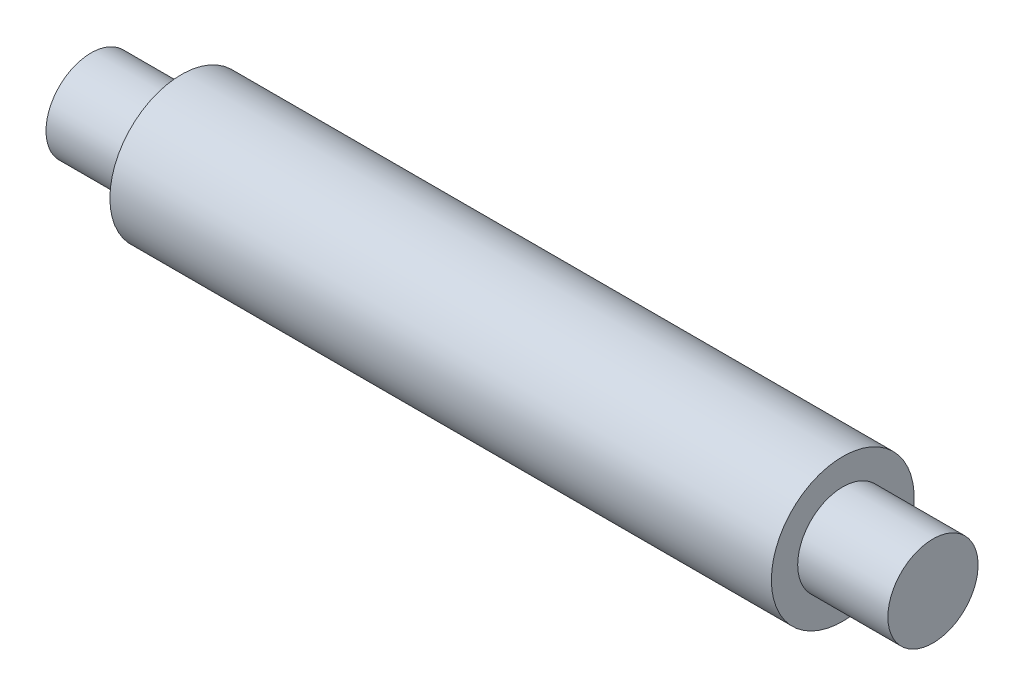
SolidWorks part; units mm, degrees
material "Plain Carbon Steel"
ref_plane "Front Plane" through (0, 0, 0) normal (0, 0, 1) x (1, 0, 0)
ref_plane "Top Plane" through (0, 0, 0) normal (0, 1, 0) x (1, 0, 0)
ref_plane "Right Plane" through (0, 0, 0) normal (1, 0, 0) x (0, 0, -1)
sketch "Roller Profile Sketch" plane through (0, 0, 0) normal (0, 0, 1) x (1, 0, 0)
  line L0 (-409.6163, 0) -> (372.6449, 0)
  line L1 (220, 47.5) -> (-220, 47.5)
  line L2 (220, 47.5) -> (220, 30)
  line L4 (-220, 47.5) -> (-220, 30)
  line L7 (-220, 30) -> (-280, 30)
  line L10 (-280, 30) -> (-280, 0)
  line L13 (280, 30) -> (220, 30)
  line L14 (280, 30) -> (280, 0)
  point P0 (0, 0)
  point P6 (-220, 0)
  point P11 (220, 0)
  dimension "D1" = 440
  dimension "D2" = 60
  dimension "D3" = 280
  dimension "D4" = 60
  dimension "D5" = 652.6449
  dimension "D6" = 129.6163
  dimension "D7" = 30
  dimension "D8" = 47.5
revolve "Roller Body Thin Revolve" add sketch "Roller Profile Sketch" angle 360 about L0
